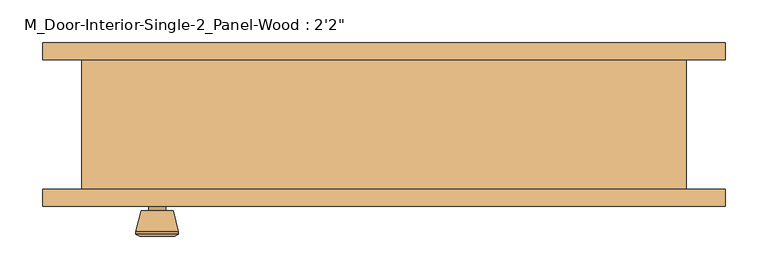
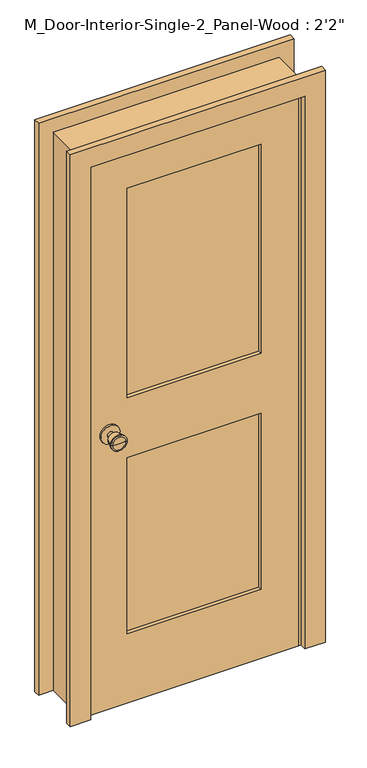
"""IFC4 building model written with IfcOpenShell, lengths in millimetres: door geometry."""

from ifc_helpers import new_model, si_unit, point, frame, frame_2d, origin, place, context, project, spatial, polyline, circle_curve, trimmed, segment, composite_curve, outline, extrude, faceted_brep, source, transform, mapped, element, save
from ifc_brep_helpers import plane_surface, cylinder_surface, revolved_surface, advanced_brep


def door_c5a180fb(model_context):
    return source(origin(), model_context, "Body", "SolidModel", [
        advanced_brep(
        [(-266.7, -32.025, 914.4), (-276.7, -32.025, 914.4), (-256.7, -32.025, 914.4), (-246.2241324, 16.975, 914.4), (-287.1758676, 16.975, 914.4), (-266.7, 16.975, 914.4), (-241.7, 15.1471319, 914.4), (-291.7, 15.1471319, 914.4), (-241.7, 11.6834537, 914.4), (-291.7, 11.6834537, 914.4), (-248.063764, -13.025, 914.4), (-285.336236, -13.025, 914.4), (-256.7, -13.025, 914.4), (-276.7, -13.025, 914.4)],
        [
            (0, 1),
            (1, 2, circle_curve(frame((-266.7, -32.025, 914.4), z_axis=(0.0, -1.0, 0.0), x_axis=(-1.0, 0.0, 0.0)), 10.0)),
            (2, 0),
            (2, 1, circle_curve(frame((-266.7, -32.025, 914.4), z_axis=(0.0, -1.0, 0.0), x_axis=(-1.0, 0.0, 0.0)), 10.0)),
            (3, 4, circle_curve(frame((-266.7, 16.975, 914.4), z_axis=(0.0, 1.0, 0.0), x_axis=(-1.0, 0.0, 0.0)), 20.4758676)),
            (4, 5),
            (5, 3),
            (4, 3, circle_curve(frame((-266.7, 16.975, 914.4), z_axis=(0.0, 1.0, 0.0), x_axis=(-1.0, 0.0, 0.0)), 20.4758676)),
            (6, 7, circle_curve(frame((-266.7, 15.1471319, 914.4), z_axis=(0.0, 1.0, 0.0), x_axis=(-1.0, 0.0, 0.0)), 25.0)),
            (7, 4),
            (3, 6),
            (7, 6, circle_curve(frame((-266.7, 15.1471319, 914.4), z_axis=(0.0, 1.0, 0.0), x_axis=(-1.0, 0.0, 0.0)), 25.0)),
            (8, 9, circle_curve(frame((-266.7, 11.6834537, 914.4), z_axis=(0.0, 1.0, 0.0), x_axis=(-1.0, 0.0, 0.0)), 25.0)),
            (9, 7),
            (6, 8),
            (9, 8, circle_curve(frame((-266.7, 11.6834537, 914.4), z_axis=(0.0, 1.0, 0.0), x_axis=(-1.0, 0.0, 0.0)), 25.0)),
            (10, 11, circle_curve(frame((-266.7, -13.025, 914.4), z_axis=(0.0, 1.0, 0.0), x_axis=(-1.0, 0.0, 0.0)), 18.636236)),
            (11, 9),
            (8, 10),
            (11, 10, circle_curve(frame((-266.7, -13.025, 914.4), z_axis=(0.0, 1.0, 0.0), x_axis=(-1.0, 0.0, 0.0)), 18.636236)),
            (12, 13, circle_curve(frame((-266.7, -13.025, 914.4), z_axis=(0.0, 1.0, 0.0), x_axis=(-1.0, 0.0, 0.0)), 10.0)),
            (13, 11),
            (10, 12),
            (13, 12, circle_curve(frame((-266.7, -13.025, 914.4), z_axis=(0.0, 1.0, 0.0), x_axis=(-1.0, 0.0, 0.0)), 10.0)),
            (1, 13),
            (12, 2),
        ],
        [
            plane_surface(frame((-266.7, -32.025, 914.4), z_axis=(0.0, -1.0, 0.0), x_axis=(-1.0, 0.0, 0.0))),
            plane_surface(frame((-266.7, 16.975, 914.4), z_axis=(0.0, 1.0, 0.0), x_axis=(-1.0, 0.0, 0.0))),
            revolved_surface(polyline([(-287.1758676, 16.975, 914.4), (-291.7, 15.1471319, 914.4)]), (-266.7, -32.025, 914.4), (0.0, -1.0, 0.0)),
            cylinder_surface(frame((-266.7, -32.025, 914.4), z_axis=(0.0, -1.0, 0.0), x_axis=(-1.0, 0.0, 0.0)), 25.0),
            revolved_surface(polyline([(-291.7, 11.6834537, 914.4), (-285.336236, -13.025, 914.4)]), (-266.7, -32.025, 914.4), (0.0, -1.0, 0.0)),
            plane_surface(frame((-266.7, -13.025, 914.4), z_axis=(0.0, -1.0, 0.0), x_axis=(-1.0, 0.0, 0.0))),
            cylinder_surface(frame((-266.7, -32.025, 914.4), z_axis=(0.0, -1.0, 0.0), x_axis=(-1.0, 0.0, 0.0)), 10.0),
        ],
        [
            (0, [[1, 2, 3]]),
            (0, [[-3, 4, -1]]),
            (1, [[5, 6, 7]]),
            (1, [[8, -7, -6]]),
            (2, [[9, 10, -5, 11]]),
            (2, [[12, -11, -8, -10]]),
            (3, [[13, 14, -9, 15]]),
            (3, [[16, -15, -12, -14]]),
            (4, [[17, 18, -13, 19]]),
            (4, [[20, -19, -16, -18]]),
            (5, [[21, 22, -17, 23]]),
            (5, [[24, -23, -20, -22]]),
            (6, [[-2, 25, -21, 26]]),
            (6, [[-4, -26, -24, -25]]),
        ],
    ),
        extrude(outline(composite_curve([segment(trimmed(circle_curve(frame_2d((914.4, -266.7)), 30.0), [point((914.4, -296.7))], [point((914.4, -236.7))], False, "CARTESIAN"), True, "CONTINUOUS"), segment(trimmed(circle_curve(frame_2d((914.4, -266.7)), 30.0), [point((914.4, -236.7))], [point((914.4, -296.7))], False, "CARTESIAN"), True, "CONTINUOUS")], self_intersect=False)), frame((0.0, -38.025, 0.0), z_axis=(0.0, 1.0, 0.0), x_axis=(0.0, 0.0, 1.0)), (0.0, 0.0, 1.0), 6.0),
        advanced_brep(
        [(-266.7, -79.025, 914.4), (-256.7, -79.025, 914.4), (-276.7, -79.025, 914.4), (-246.2241324, -128.025, 914.4), (-266.7, -128.025, 914.4), (-287.1758676, -128.025, 914.4), (-241.7, -126.1971319, 914.4), (-291.7, -126.1971319, 914.4), (-241.7, -122.7334537, 914.4), (-291.7, -122.7334537, 914.4), (-248.063764, -98.025, 914.4), (-285.336236, -98.025, 914.4), (-256.7, -98.025, 914.4), (-276.7, -98.025, 914.4)],
        [
            (0, 1),
            (1, 2, circle_curve(frame((-266.7, -79.025, 914.4), z_axis=(0.0, 1.0, 0.0), x_axis=(-1.0, 0.0, 0.0)), 10.0)),
            (2, 0),
            (2, 1, circle_curve(frame((-266.7, -79.025, 914.4), z_axis=(0.0, 1.0, 0.0), x_axis=(-1.0, 0.0, 0.0)), 10.0)),
            (3, 4),
            (4, 5),
            (5, 3, circle_curve(frame((-266.7, -128.025, 914.4), z_axis=(0.0, -1.0, 0.0), x_axis=(-1.0, 0.0, 0.0)), 20.4758676)),
            (3, 5, circle_curve(frame((-266.7, -128.025, 914.4), z_axis=(0.0, -1.0, 0.0), x_axis=(-1.0, 0.0, 0.0)), 20.4758676)),
            (6, 3),
            (5, 7),
            (7, 6, circle_curve(frame((-266.7, -126.1971319, 914.4), z_axis=(0.0, -1.0, 0.0), x_axis=(-1.0, 0.0, 0.0)), 25.0)),
            (6, 7, circle_curve(frame((-266.7, -126.1971319, 914.4), z_axis=(0.0, -1.0, 0.0), x_axis=(-1.0, 0.0, 0.0)), 25.0)),
            (8, 6),
            (7, 9),
            (9, 8, circle_curve(frame((-266.7, -122.7334537, 914.4), z_axis=(0.0, -1.0, 0.0), x_axis=(-1.0, 0.0, 0.0)), 25.0)),
            (8, 9, circle_curve(frame((-266.7, -122.7334537, 914.4), z_axis=(0.0, -1.0, 0.0), x_axis=(-1.0, 0.0, 0.0)), 25.0)),
            (10, 8),
            (9, 11),
            (11, 10, circle_curve(frame((-266.7, -98.025, 914.4), z_axis=(0.0, -1.0, 0.0), x_axis=(-1.0, 0.0, 0.0)), 18.636236)),
            (10, 11, circle_curve(frame((-266.7, -98.025, 914.4), z_axis=(0.0, -1.0, 0.0), x_axis=(-1.0, 0.0, 0.0)), 18.636236)),
            (12, 10),
            (11, 13),
            (13, 12, circle_curve(frame((-266.7, -98.025, 914.4), z_axis=(0.0, -1.0, 0.0), x_axis=(-1.0, 0.0, 0.0)), 10.0)),
            (12, 13, circle_curve(frame((-266.7, -98.025, 914.4), z_axis=(0.0, -1.0, 0.0), x_axis=(-1.0, 0.0, 0.0)), 10.0)),
            (1, 12),
            (13, 2),
        ],
        [
            plane_surface(frame((-266.7, -79.025, 914.4), z_axis=(0.0, 1.0, 0.0), x_axis=(-1.0, 0.0, 0.0))),
            plane_surface(frame((-266.7, -128.025, 914.4), z_axis=(0.0, -1.0, 0.0), x_axis=(-1.0, 0.0, 0.0))),
            revolved_surface(polyline([(-287.1758676, -128.025, 914.4), (-291.7, -126.1971319, 914.4)]), (-266.7, -79.025, 914.4), (0.0, 1.0, 0.0)),
            cylinder_surface(frame((-266.7, -79.025, 914.4), z_axis=(0.0, 1.0, 0.0), x_axis=(-1.0, 0.0, 0.0)), 25.0),
            revolved_surface(polyline([(-291.7, -122.7334537, 914.4), (-285.336236, -98.025, 914.4)]), (-266.7, -79.025, 914.4), (0.0, 1.0, 0.0)),
            plane_surface(frame((-266.7, -98.025, 914.4), z_axis=(0.0, 1.0, 0.0), x_axis=(-1.0, 0.0, 0.0))),
            cylinder_surface(frame((-266.7, -79.025, 914.4), z_axis=(0.0, 1.0, 0.0), x_axis=(-1.0, 0.0, 0.0)), 10.0),
        ],
        [
            (0, [[1, 2, 3]]),
            (0, [[-3, 4, -1]]),
            (1, [[5, 6, 7]]),
            (1, [[-6, -5, 8]]),
            (2, [[9, -7, 10, 11]]),
            (2, [[-10, -8, -9, 12]]),
            (3, [[13, -11, 14, 15]]),
            (3, [[-14, -12, -13, 16]]),
            (4, [[17, -15, 18, 19]]),
            (4, [[-18, -16, -17, 20]]),
            (5, [[21, -19, 22, 23]]),
            (5, [[-22, -20, -21, 24]]),
            (6, [[25, -23, 26, -2]]),
            (6, [[-26, -24, -25, -4]]),
        ],
    ),
        extrude(outline(composite_curve([segment(trimmed(circle_curve(frame_2d((914.4, -266.7)), 30.0), [point((914.4, -296.7))], [point((914.4, -236.7))], False, "CARTESIAN"), True, "CONTINUOUS"), segment(trimmed(circle_curve(frame_2d((914.4, -266.7)), 30.0), [point((914.4, -236.7))], [point((914.4, -296.7))], False, "CARTESIAN"), True, "CONTINUOUS")], self_intersect=False)), frame((0.0, -79.025, 0.0), z_axis=(0.0, 1.0, 0.0), x_axis=(0.0, 0.0, 1.0)), (0.0, 0.0, 1.0), 6.0),
        faceted_brep([(355.2, -73.025, 0.0), (330.2, -73.025, 0.0), (330.2, -38.025, 0.0), (317.5, -38.025, 0.0), (317.5, -3.1, 0.0), (330.2, -3.1, 0.0), (330.2, 79.375, 0.0), (355.2, 79.375, 0.0), (355.2, 79.375, 1853.8), (355.2, -73.025, 1853.8), (330.2, 79.375, 1828.8), (-330.2, 79.375, 1828.8), (-330.2, 79.375, 0.0), (-355.2, 79.375, 0.0), (-355.2, 79.375, 1853.8), (330.2, -3.1, 1828.8), (317.5, -3.1, 1816.1), (-317.5, -3.1, 1816.1), (-317.5, -3.1, 0.0), (-330.2, -3.1, 0.0), (-330.2, -3.1, 1828.8), (317.5, -38.025, 1816.1), (330.2, -38.025, 1828.8), (-330.2, -38.025, 1828.8), (-330.2, -38.025, 0.0), (-317.5, -38.025, 0.0), (-317.5, -38.025, 1816.1), (330.2, -73.025, 1828.8), (-355.2, -73.025, 1853.8), (-355.2, -73.025, 0.0), (-330.2, -73.025, 0.0), (-330.2, -73.025, 1828.8)], [[[0, 1, 2, 3, 4, 5, 6, 7]], [[7, 8, 9, 0]], [[6, 10, 11, 12, 13, 14, 8, 7]], [[5, 15, 10, 6]], [[4, 16, 17, 18, 19, 20, 15, 5]], [[3, 21, 16, 4]], [[2, 22, 23, 24, 25, 26, 21, 3]], [[1, 27, 22, 2]], [[0, 9, 28, 29, 30, 31, 27, 1]], [[8, 14, 28, 9]], [[15, 20, 11, 10]], [[21, 26, 17, 16]], [[27, 31, 23, 22]], [[29, 13, 12, 19, 18, 25, 24, 30]], [[14, 13, 29, 28]], [[20, 19, 12, 11]], [[26, 25, 18, 17]], [[31, 30, 24, 23]]]),
        extrude(outline(polyline([(1828.8, -330.2), (0.0, -330.2), (0.0, 330.2), (1828.8, 330.2), (1828.8, -330.2)]), holes=[polyline([(1708.8, -210.2), (1708.8, 210.2), (1014.4, 210.2), (1014.4, -210.2), (1708.8, -210.2)]), polyline([(814.4, -210.2), (814.4, 210.2), (230.0, 210.2), (230.0, -210.2), (814.4, -210.2)])]), frame((0.0, -73.025, 0.0), z_axis=(0.0, 1.0, 0.0), x_axis=(0.0, 0.0, 1.0)), (0.0, 0.0, 1.0), 35.0),
        extrude(outline(polyline([(210.2, -49.6916667), (210.2, -61.3583333), (-210.2, -61.3583333), (-210.2, -49.6916667), (210.2, -49.6916667)])), frame((0.0, 0.0, 1014.4), z_axis=(0.0, 0.0, 1.0), x_axis=(1.0, 0.0, 0.0)), (0.0, 0.0, 1.0), 694.4),
        extrude(outline(polyline([(210.2, -49.6916667), (210.2, -61.3583333), (-210.2, -61.3583333), (-210.2, -49.6916667), (210.2, -49.6916667)])), frame((0.0, 0.0, 230.0), z_axis=(0.0, 0.0, 1.0), x_axis=(1.0, 0.0, 0.0)), (0.0, 0.0, 1.0), 584.4),
        extrude(outline(polyline([(0.0, 401.55), (1900.15, 401.55), (1900.15, -401.55), (0.0, -401.55), (0.0, -336.55), (1835.15, -336.55), (1835.15, 336.55), (0.0, 336.55), (0.0, 401.55)])), frame((0.0, -93.025, 0.0), z_axis=(0.0, 1.0, 0.0), x_axis=(0.0, 0.0, 1.0)), (0.0, 0.0, 1.0), 20.0),
        extrude(outline(polyline([(0.0, 401.55), (1900.15, 401.55), (1900.15, -401.55), (0.0, -401.55), (0.0, -336.55), (1835.15, -336.55), (1835.15, 336.55), (0.0, 336.55), (0.0, 401.55)])), frame((0.0, 79.375, 0.0), z_axis=(0.0, 1.0, 0.0), x_axis=(0.0, 0.0, 1.0)), (0.0, 0.0, 1.0), 20.0),
    ])


if __name__ == "__main__":
    model = new_model("IFC4")
    model_context = context("Model", 3, world=origin())
    ifc_project = project(units=[si_unit("LENGTHUNIT", "METRE", prefix="MILLI")], contexts=[model_context])
    site = spatial("IfcSite", under=ifc_project)
    building = spatial("IfcBuilding", under=site)
    placement = place(None, origin())
    door_shape = door_c5a180fb(model_context)
    element("IfcDoor", 1, ObjectType="M_Door-Interior-Single-2_Panel-Wood : 2'2\"", at=placement, inside=building, context=model_context, shape_type="MappedRepresentation", body=[
        mapped(door_shape, transform((0.0, 0.0, 0.0), x_axis=(1.0, 0.0, 0.0), y_axis=(0.0, 1.0, 0.0), z_axis=(0.0, 0.0, 1.0))),
    ])
    save(model, "model.ifc")

# Revit data of these elements
# Type "M_Door-Interior-Single-2_Panel-Wood : 2'2\""
#   Type Mark = "11"
#   Assembly Code = "C1020300"
#   Analytic Construction = "Wooden"
#   Top Rail = 0' - 4.72441"
#   Thickness = 0' - 1.37795"
#   Thermal Resistance (R) = 2.5876 (h·ft²·°F)/BTU
#   Swing Angle [instance default] = 90.00°
#   Stiles = 0' - 4.72441"
#   Rough Width = 2' - 3.9685"
#   Rough Height = 6' - 0.98425"
#   Lock Rail = 0' - 7.87402"
#   Height = 6' - 0"
#   Width = 2' - 2"
#   Heat Transfer Coefficient (U) = 0.3865 BTU/(h·ft²·°F)
#   Bottom Rail = 0' - 9.05512"
#   Trim Material = Cherry
#   Panel Material = Cherry
#   Frame Material = Cherry
#   Door Handle Material = Aluminum
#   Visual Light Transmittance = 0
#   Solar Heat Gain Coefficient = 0
#   Wall Closure = (empty or 0)
#   Function = (empty or 0)
# Element 1 (IfcDoor, "M_Door-Interior-Single-2_Panel-Wood : 2'2\"")
#   Materials on its faces: "Cherry", "Aluminum"
# Materials
#   "Cherry": class "Wood", colour RGB 226 177 128, transparency 0, Description = "Prunus Serotina", Cost = 0
#   "Aluminum": class "Metal", colour RGB 247 247 247, transparency 0, Description = "Aluminum 6061", Cost = 0
